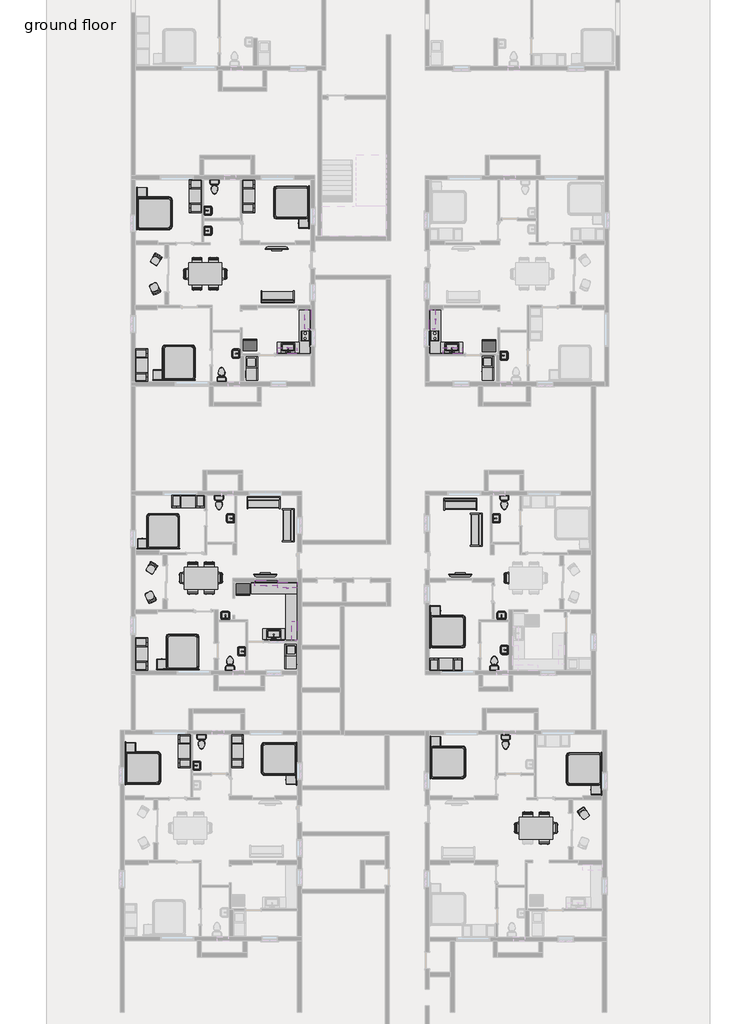
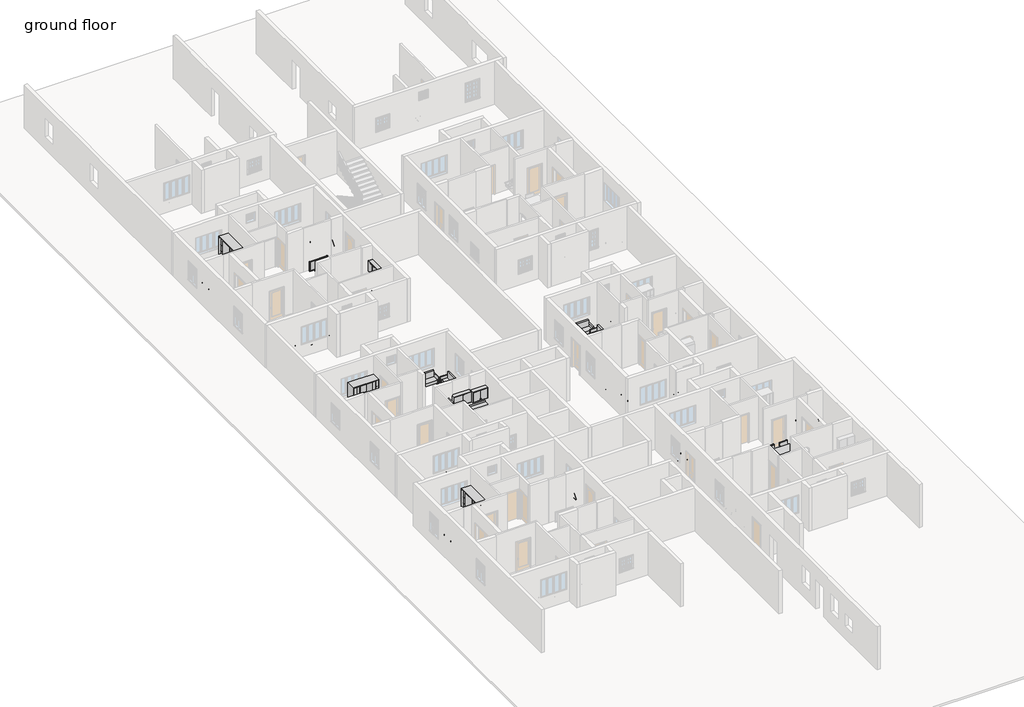
# One storey, part 12 of 16: 77 furniture elements, 22 flow terminals, 11 proxies.
"""IFC4 building model written with IfcOpenShell, lengths in millimetres."""

from ifc_helpers import new_model, si_unit, origin, place, context, project, spatial, transform, mapped, element, save
from components import proxy_84368fe0, proxy_40295e01, proxy_97c73763, proxy_19935bb1, proxy_76352e5b, proxy_1934c8a4, flow_terminal_4d548711, flow_terminal_3ac2e542, flow_terminal_8d9ea526, toilet_domestic_3d_toilet_domestic_3d_ba6479b0, toilet_domestic_3d_toilet_domestic_3d_30431060, bed_design_8999_bed_design_8999_9c973422, bed_design_8999_bed_design_8999_e911dec7, furniture_f87f75a4, furniture_a56de0b1, furniture_5f863b49, furniture_6369f5ad, furniture_97fe820d, furniture_007fecef, chair_task_chair_task_b7f3823b, chair_task_arms_chair_task_arms_fa5a08ef, furniture_deb1c5d1, furniture_78fcf777, furniture_90663022, furniture_1a836c3b, furniture_8d0dc8c9, furniture_49e6720b, furniture_88072bd9, furniture_eb3a3c23, furniture_4fdbbe14, furniture_57f9710a, furniture_0b81fedb, furniture_0bcc43ae, furniture_9929ec1f, furniture_f73e1c42, furniture_4a8f7e85

model = new_model("IFC4")

# Units and contexts
model_context = context("Model", 3, world=origin())
ifc_project = project(units=[si_unit("LENGTHUNIT", "METRE", prefix="MILLI")], contexts=[model_context])

# Site, building, storey
site = spatial("IfcSite", under=ifc_project)
building = spatial("IfcBuilding", under=site)
storey = spatial("IfcBuildingStorey", under=building, Name="ground floor", Elevation=609.6)

# Proxies
placement = place(None, origin())
proxy_shape = proxy_84368fe0(model_context)
element("IfcBuildingElementProxy", 1, Name="Cook Top-2 Unit : 16\" x 22\"", ObjectType="Cook Top-2 Unit : 16\" x 22\"", at=placement, inside=storey, context=model_context, shape_type="MappedRepresentation", body=[
    mapped(proxy_shape, transform((52653.926243, 23760.8750503, 609.6), x_axis=(1.0, 0.0, 0.0), y_axis=(0.0, 1.0, 0.0), z_axis=(0.0, 0.0, 1.0))),
])
proxy_2_shape = proxy_40295e01(model_context)
element("IfcBuildingElementProxy", 2, Name="Cook Top-2 Unit : 16\" x 22\"", ObjectType="Cook Top-2 Unit : 16\" x 22\"", at=placement, inside=storey, context=model_context, shape_type="MappedRepresentation", body=[
    mapped(proxy_2_shape, transform((59966.1312819, 23760.8750503, 609.6), x_axis=(-1.0, 0.0, 0.0), y_axis=(0.0, -1.0, 0.0), z_axis=(0.0, 0.0, 1.0))),
])
proxy_3_shape = proxy_97c73763(model_context)
element("IfcBuildingElementProxy", 3, Name="Dryer : 27\" x 25\" x 35\"", ObjectType="Dryer : 27\" x 25\" x 35\"", at=placement, inside=storey, context=model_context, shape_type="MappedRepresentation", body=[
    mapped(proxy_3_shape, transform((62510.7278279, 22075.5934981, 609.6), x_axis=(0.0, -1.0, 0.0), y_axis=(1.0, 0.0, 0.0), z_axis=(0.0, 0.0, 1.0))),
])
element("IfcBuildingElementProxy", 4, Name="Dryer : 27\" x 25\" x 35\"", ObjectType="Dryer : 27\" x 25\" x 35\"", at=placement, inside=storey, context=model_context, shape_type="MappedRepresentation", body=[
    mapped(proxy_3_shape, transform((49480.5278279, 22050.1934981, 609.6), x_axis=(0.0, -1.0, 0.0), y_axis=(1.0, 0.0, 0.0), z_axis=(0.0, 0.0, 1.0))),
])
element("IfcBuildingElementProxy", 5, Name="Dryer : 27\" x 25\" x 35\"", ObjectType="Dryer : 27\" x 25\" x 35\"", at=placement, inside=storey, context=model_context, shape_type="MappedRepresentation", body=[
    mapped(proxy_3_shape, transform((52244.3504974, 5396.4843277, 609.6), x_axis=(0.0, 1.0, 0.0), y_axis=(-1.0, 0.0, 0.0), z_axis=(0.0, 0.0, 1.0))),
])
proxy_4_shape = proxy_19935bb1(model_context)
element("IfcBuildingElementProxy", 6, Name="Refrigerator-Built-in : 30\" x 24\" LH", ObjectType="Refrigerator-Built-in : 30\" x 24\" LH", at=placement, inside=storey, context=model_context, shape_type="MappedRepresentation", body=[
    mapped(proxy_4_shape, transform((49314.0778826, 9828.1563876, 609.6), x_axis=(1.0, 0.0, 0.0), y_axis=(0.0, 1.0, 0.0), z_axis=(0.0, 0.0, 1.0))),
])
proxy_5_shape = proxy_76352e5b(model_context)
element("IfcBuildingElementProxy", 7, Name="Refrigerator-Built-in : 30\" x 24\" LH", ObjectType="Refrigerator-Built-in : 30\" x 24\" LH", at=placement, inside=storey, context=model_context, shape_type="MappedRepresentation", body=[
    mapped(proxy_5_shape, transform((62882.4552131, 23205.265558, 609.6), x_axis=(1.0, 0.0, 0.0), y_axis=(0.0, 1.0, 0.0), z_axis=(0.0, 0.0, 1.0))),
])
element("IfcBuildingElementProxy", 8, Name="Refrigerator-Built-in : 30\" x 24\" LH", ObjectType="Refrigerator-Built-in : 30\" x 24\" LH", at=placement, inside=storey, context=model_context, shape_type="MappedRepresentation", body=[
    mapped(proxy_5_shape, transform((49699.8552131, 23256.065558, 609.6), x_axis=(1.0, 0.0, 0.0), y_axis=(0.0, 1.0, 0.0), z_axis=(0.0, 0.0, 1.0))),
])
proxy_6_shape = proxy_1934c8a4(model_context)
element("IfcBuildingElementProxy", 9, Name="Washer : 25\" x 25\" x 35\"", ObjectType="Washer : 25\" x 25\" x 35\"", at=placement, inside=storey, context=model_context, shape_type="MappedRepresentation", body=[
    mapped(proxy_6_shape, transform((62546.2392669, 22752.0235103, 609.6), x_axis=(0.0, -1.0, 0.0), y_axis=(1.0, 0.0, 0.0), z_axis=(0.0, 0.0, 1.0))),
])
element("IfcBuildingElementProxy", 10, Name="Washer : 25\" x 25\" x 35\"", ObjectType="Washer : 25\" x 25\" x 35\"", at=placement, inside=storey, context=model_context, shape_type="MappedRepresentation", body=[
    mapped(proxy_6_shape, transform((49516.0392669, 22726.6235103, 609.6), x_axis=(0.0, -1.0, 0.0), y_axis=(1.0, 0.0, 0.0), z_axis=(0.0, 0.0, 1.0))),
])
element("IfcBuildingElementProxy", 11, Name="Washer : 25\" x 25\" x 35\"", ObjectType="Washer : 25\" x 25\" x 35\"", at=placement, inside=storey, context=model_context, shape_type="MappedRepresentation", body=[
    mapped(proxy_6_shape, transform((52203.6619364, 6072.9143399, 609.6), x_axis=(0.0, 1.0, 0.0), y_axis=(-1.0, 0.0, 0.0), z_axis=(0.0, 0.0, 1.0))),
])

# Flow terminals
flow_terminal_shape = flow_terminal_4d548711(model_context)
element("IfcFlowTerminal", 12, ObjectType="Sink Kitchen-Single : 30\" x 21\"", at=placement, inside=storey, context=model_context, shape_type="MappedRepresentation", body=[
    mapped(flow_terminal_shape, transform((51806.0154836, 23119.0104663, 609.6), x_axis=(-1.0, 0.0, 0.0), y_axis=(0.0, -1.0, 0.0), z_axis=(0.0, 0.0, 1.0))),
])
element("IfcFlowTerminal", 13, ObjectType="Sink Kitchen-Single : 30\" x 21\"", at=placement, inside=storey, context=model_context, shape_type="MappedRepresentation", body=[
    mapped(flow_terminal_shape, transform((51016.5809161, 7307.5104663, 609.6), x_axis=(-1.0, 0.0, 0.0), y_axis=(0.0, -1.0, 0.0), z_axis=(0.0, 0.0, 1.0))),
])
flow_terminal_2_shape = flow_terminal_3ac2e542(model_context)
element("IfcFlowTerminal", 14, ObjectType="Sink Kitchen-Single : 30\" x 21\"", at=placement, inside=storey, context=model_context, shape_type="MappedRepresentation", body=[
    mapped(flow_terminal_2_shape, transform((60814.0420413, 23119.0104663, 609.6), x_axis=(1.0, 0.0, 0.0), y_axis=(0.0, 1.0, 0.0), z_axis=(0.0, 0.0, 1.0))),
])
flow_terminal_3_shape = flow_terminal_8d9ea526(model_context)
element("IfcFlowTerminal", 15, ObjectType="Sink Vanity-Square : 20\" x 18\"", at=placement, inside=storey, context=model_context, shape_type="MappedRepresentation", body=[
    mapped(flow_terminal_3_shape, transform((63651.476683, 22681.8758246, 609.6), x_axis=(0.0, 1.0, 0.0), y_axis=(-1.0, 0.0, 0.0), z_axis=(0.0, 0.0, 1.0))),
])
element("IfcFlowTerminal", 16, ObjectType="Sink Vanity-Square : 20\" x 18\"", at=placement, inside=storey, context=model_context, shape_type="MappedRepresentation", body=[
    mapped(flow_terminal_3_shape, transform((63232.376683, 13706.0559785, 609.6), x_axis=(0.0, 1.0, 0.0), y_axis=(-1.0, 0.0, 0.0), z_axis=(0.0, 0.0, 1.0))),
])
element("IfcFlowTerminal", 17, ObjectType="Sink Vanity-Square : 20\" x 18\"", at=placement, inside=storey, context=model_context, shape_type="MappedRepresentation", body=[
    mapped(flow_terminal_3_shape, transform((63582.2705224, 8323.5104663, 609.6), x_axis=(-1.0, 0.0, 0.0), y_axis=(0.0, -1.0, 0.0), z_axis=(0.0, 0.0, 1.0))),
])
element("IfcFlowTerminal", 18, ObjectType="Sink Vanity-Square : 20\" x 18\"", at=placement, inside=storey, context=model_context, shape_type="MappedRepresentation", body=[
    mapped(flow_terminal_3_shape, transform((63773.7858807, 6482.6543057, 609.6), x_axis=(0.0, -1.0, 0.0), y_axis=(1.0, 0.0, 0.0), z_axis=(0.0, 0.0, 1.0))),
])
element("IfcFlowTerminal", 19, ObjectType="Sink Vanity-Square : 20\" x 18\"", at=placement, inside=storey, context=model_context, shape_type="MappedRepresentation", body=[
    mapped(flow_terminal_3_shape, transform((46712.6716441, 66.9997113, 609.6), x_axis=(0.0, 1.0, 0.0), y_axis=(-1.0, 0.0, 0.0), z_axis=(0.0, 0.0, 1.0))),
])
element("IfcFlowTerminal", 20, ObjectType="Sink Vanity-Square : 20\" x 18\"", at=placement, inside=storey, context=model_context, shape_type="MappedRepresentation", body=[
    mapped(flow_terminal_3_shape, transform((49283.8822894, 6399.086689, 609.6), x_axis=(-0.012057146916581555, -0.9999273099621953, 0.0), y_axis=(0.9999273099621953, -0.012057146916581555, 0.0), z_axis=(0.0, 0.0, 1.0))),
])
element("IfcFlowTerminal", 21, ObjectType="Sink Vanity-Square : 20\" x 18\"", at=placement, inside=storey, context=model_context, shape_type="MappedRepresentation", body=[
    mapped(flow_terminal_3_shape, transform((48351.6154836, 8323.5104663, 609.6), x_axis=(-1.0, 0.0, 0.0), y_axis=(0.0, -1.0, 0.0), z_axis=(0.0, 0.0, 1.0))),
])
element("IfcFlowTerminal", 22, ObjectType="Sink Vanity-Square : 20\" x 18\"", at=placement, inside=storey, context=model_context, shape_type="MappedRepresentation", body=[
    mapped(flow_terminal_3_shape, transform((48663.7808419, 13737.4344596, 609.6), x_axis=(0.0, -1.0, 0.0), y_axis=(1.0, 0.0, 0.0), z_axis=(0.0, 0.0, 1.0))),
])
element("IfcFlowTerminal", 23, ObjectType="Sink Vanity-Square : 20\" x 18\"", at=placement, inside=storey, context=model_context, shape_type="MappedRepresentation", body=[
    mapped(flow_terminal_3_shape, transform((48968.5808419, 22827.5543057, 609.6), x_axis=(0.0, -1.0, 0.0), y_axis=(1.0, 0.0, 0.0), z_axis=(0.0, 0.0, 1.0))),
])
element("IfcFlowTerminal", 24, ObjectType="Sink Vanity-Square : 20\" x 18\"", at=placement, inside=storey, context=model_context, shape_type="MappedRepresentation", body=[
    mapped(flow_terminal_3_shape, transform((47322.2716441, 29569.0881062, 609.6), x_axis=(0.0, 1.0, 0.0), y_axis=(-1.0, 0.0, 0.0), z_axis=(0.0, 0.0, 1.0))),
])
element("IfcFlowTerminal", 25, ObjectType="Sink Vanity-Square : 20\" x 18\"", at=placement, inside=storey, context=model_context, shape_type="MappedRepresentation", body=[
    mapped(flow_terminal_3_shape, transform((47322.2716441, 30681.1004564, 609.6), x_axis=(0.0, 1.0, 0.0), y_axis=(-1.0, 0.0, 0.0), z_axis=(0.0, 0.0, 1.0))),
])
toilet_domestic_3d_toilet_domestic_3d_shape = toilet_domestic_3d_toilet_domestic_3d_ba6479b0(model_context)
toilet_domestic_3d_toilet_domestic_3d_2_shape = toilet_domestic_3d_toilet_domestic_3d_30431060(model_context)
element("IfcFlowTerminal", 26, ObjectType="Toilet-Domestic-3D : Toilet-Domestic-3D", at=placement, inside=storey, context=model_context, shape_type="MappedRepresentation", body=[
    mapped(toilet_domestic_3d_toilet_domestic_3d_shape, transform((48129.1248418, 21744.3232288, 609.6), x_axis=(-1.0, 0.0, 0.0), y_axis=(0.0, -1.0, 0.0), z_axis=(0.0, 0.0, 1.0))),
    mapped(toilet_domestic_3d_toilet_domestic_3d_2_shape, transform((48129.1248418, 21744.3232288, 609.6), x_axis=(-1.0, 0.0, 0.0), y_axis=(0.0, -1.0, 0.0), z_axis=(0.0, 0.0, 1.0))),
])
element("IfcFlowTerminal", 27, ObjectType="Toilet-Domestic-3D : Toilet-Domestic-3D", at=placement, inside=storey, context=model_context, shape_type="MappedRepresentation", body=[
    mapped(toilet_domestic_3d_toilet_domestic_3d_shape, transform((47732.676243, 31918.2311741, 609.6), x_axis=(1.0, 0.0, 0.0), y_axis=(0.0, 1.0, 0.0), z_axis=(0.0, 0.0, 1.0))),
    mapped(toilet_domestic_3d_toilet_domestic_3d_2_shape, transform((47732.676243, 31918.2311741, 609.6), x_axis=(1.0, 0.0, 0.0), y_axis=(0.0, 1.0, 0.0), z_axis=(0.0, 0.0, 1.0))),
])
element("IfcFlowTerminal", 28, ObjectType="Toilet-Domestic-3D : Toilet-Domestic-3D", at=placement, inside=storey, context=model_context, shape_type="MappedRepresentation", body=[
    mapped(toilet_domestic_3d_toilet_domestic_3d_shape, transform((47986.676243, 14503.375789, 609.6), x_axis=(1.0, 0.0, 0.0), y_axis=(0.0, 1.0, 0.0), z_axis=(0.0, 0.0, 1.0))),
    mapped(toilet_domestic_3d_toilet_domestic_3d_2_shape, transform((47986.676243, 14503.375789, 609.6), x_axis=(1.0, 0.0, 0.0), y_axis=(0.0, 1.0, 0.0), z_axis=(0.0, 0.0, 1.0))),
])
element("IfcFlowTerminal", 29, ObjectType="Toilet-Domestic-3D : Toilet-Domestic-3D", at=placement, inside=storey, context=model_context, shape_type="MappedRepresentation", body=[
    mapped(toilet_domestic_3d_toilet_domestic_3d_shape, transform((48589.926243, 5815.3678437, 609.6), x_axis=(-1.0, 0.0, 0.0), y_axis=(0.0, -1.0, 0.0), z_axis=(0.0, 0.0, 1.0))),
    mapped(toilet_domestic_3d_toilet_domestic_3d_2_shape, transform((48589.926243, 5815.3678437, 609.6), x_axis=(-1.0, 0.0, 0.0), y_axis=(0.0, -1.0, 0.0), z_axis=(0.0, 0.0, 1.0))),
])
element("IfcFlowTerminal", 30, ObjectType="Toilet-Domestic-3D : Toilet-Domestic-3D", at=placement, inside=storey, context=model_context, shape_type="MappedRepresentation", body=[
    mapped(toilet_domestic_3d_toilet_domestic_3d_shape, transform((63166.5312819, 5818.6610925, 609.6), x_axis=(-1.0, 0.0, 0.0), y_axis=(0.0, -1.0, 0.0), z_axis=(0.0, 0.0, 1.0))),
    mapped(toilet_domestic_3d_toilet_domestic_3d_2_shape, transform((63166.5312819, 5818.6610925, 609.6), x_axis=(-1.0, 0.0, 0.0), y_axis=(0.0, -1.0, 0.0), z_axis=(0.0, 0.0, 1.0))),
])
element("IfcFlowTerminal", 31, ObjectType="Toilet-Domestic-3D : Toilet-Domestic-3D", at=placement, inside=storey, context=model_context, shape_type="MappedRepresentation", body=[
    mapped(toilet_domestic_3d_toilet_domestic_3d_shape, transform((63718.9812819, 14506.6690378, 609.6), x_axis=(1.0, 0.0, 0.0), y_axis=(0.0, 1.0, 0.0), z_axis=(0.0, 0.0, 1.0))),
    mapped(toilet_domestic_3d_toilet_domestic_3d_2_shape, transform((63718.9812819, 14506.6690378, 609.6), x_axis=(1.0, 0.0, 0.0), y_axis=(0.0, 1.0, 0.0), z_axis=(0.0, 0.0, 1.0))),
])
element("IfcFlowTerminal", 32, ObjectType="Toilet-Domestic-3D : Toilet-Domestic-3D", at=placement, inside=storey, context=model_context, shape_type="MappedRepresentation", body=[
    mapped(toilet_domestic_3d_toilet_domestic_3d_shape, transform((63795.1812819, 1292.0926062, 609.6), x_axis=(1.0, 0.0, 0.0), y_axis=(0.0, 1.0, 0.0), z_axis=(0.0, 0.0, 1.0))),
    mapped(toilet_domestic_3d_toilet_domestic_3d_2_shape, transform((63795.1812819, 1292.0926062, 609.6), x_axis=(1.0, 0.0, 0.0), y_axis=(0.0, 1.0, 0.0), z_axis=(0.0, 0.0, 1.0))),
])
element("IfcFlowTerminal", 33, ObjectType="Toilet-Domestic-3D : Toilet-Domestic-3D", at=placement, inside=storey, context=model_context, shape_type="MappedRepresentation", body=[
    mapped(toilet_domestic_3d_toilet_domestic_3d_shape, transform((47021.476243, 1304.7926062, 609.6), x_axis=(1.0, 0.0, 0.0), y_axis=(0.0, 1.0, 0.0), z_axis=(0.0, 0.0, 1.0))),
    mapped(toilet_domestic_3d_toilet_domestic_3d_2_shape, transform((47021.476243, 1304.7926062, 609.6), x_axis=(1.0, 0.0, 0.0), y_axis=(0.0, 1.0, 0.0), z_axis=(0.0, 0.0, 1.0))),
])

# Furniture
bed_design_8999_bed_design_8999_shape = bed_design_8999_bed_design_8999_9c973422(model_context)
bed_design_8999_bed_design_8999_2_shape = bed_design_8999_bed_design_8999_e911dec7(model_context)
element("IfcFurniture", 34, ObjectType="BED_DESIGN_8999 : BED_DESIGN_8999", at=placement, inside=storey, context=model_context, shape_type="MappedRepresentation", body=[
    mapped(bed_design_8999_bed_design_8999_shape, transform((61568.6818649, 7679.8150652, 609.6), x_axis=(0.0, 1.0, 0.0), y_axis=(-1.0, 0.0, 0.0), z_axis=(0.0, 0.0, 1.0))),
    mapped(bed_design_8999_bed_design_8999_2_shape, transform((61568.6818649, 7679.8150652, 609.6), x_axis=(0.0, 1.0, 0.0), y_axis=(-1.0, 0.0, 0.0), z_axis=(0.0, 0.0, 1.0))),
])
element("IfcFurniture", 35, ObjectType="BED_DESIGN_8999 : BED_DESIGN_8999", at=placement, inside=storey, context=model_context, shape_type="MappedRepresentation", body=[
    mapped(bed_design_8999_bed_design_8999_shape, transform((67141.6312819, -302.3613664, 609.6), x_axis=(0.0, -1.0, 0.0), y_axis=(1.0, 0.0, 0.0), z_axis=(0.0, 0.0, 1.0))),
    mapped(bed_design_8999_bed_design_8999_2_shape, transform((67141.6312819, -302.3613664, 609.6), x_axis=(0.0, -1.0, 0.0), y_axis=(1.0, 0.0, 0.0), z_axis=(0.0, 0.0, 1.0))),
])
element("IfcFurniture", 36, ObjectType="BED_DESIGN_8999 : BED_DESIGN_8999", at=placement, inside=storey, context=model_context, shape_type="MappedRepresentation", body=[
    mapped(bed_design_8999_bed_design_8999_shape, transform((61579.0312819, 460.9590685, 609.6), x_axis=(0.0, 1.0, 0.0), y_axis=(-1.0, 0.0, 0.0), z_axis=(0.0, 0.0, 1.0))),
    mapped(bed_design_8999_bed_design_8999_2_shape, transform((61579.0312819, 460.9590685, 609.6), x_axis=(0.0, 1.0, 0.0), y_axis=(-1.0, 0.0, 0.0), z_axis=(0.0, 0.0, 1.0))),
])
element("IfcFurniture", 37, ObjectType="BED_DESIGN_8999 : BED_DESIGN_8999", at=placement, inside=storey, context=model_context, shape_type="MappedRepresentation", body=[
    mapped(bed_design_8999_bed_design_8999_shape, transform((44754.526243, 147.57086, 609.6), x_axis=(0.0, 1.0, 0.0), y_axis=(-1.0, 0.0, 0.0), z_axis=(0.0, 0.0, 1.0))),
    mapped(bed_design_8999_bed_design_8999_2_shape, transform((44754.526243, 147.57086, 609.6), x_axis=(0.0, 1.0, 0.0), y_axis=(-1.0, 0.0, 0.0), z_axis=(0.0, 0.0, 1.0))),
])
element("IfcFurniture", 38, ObjectType="BED_DESIGN_8999 : BED_DESIGN_8999", at=placement, inside=storey, context=model_context, shape_type="MappedRepresentation", body=[
    mapped(bed_design_8999_bed_design_8999_shape, transform((50317.126243, 256.4386336, 609.6), x_axis=(0.0, -1.0, 0.0), y_axis=(1.0, 0.0, 0.0), z_axis=(0.0, 0.0, 1.0))),
    mapped(bed_design_8999_bed_design_8999_2_shape, transform((50317.126243, 256.4386336, 609.6), x_axis=(0.0, -1.0, 0.0), y_axis=(1.0, 0.0, 0.0), z_axis=(0.0, 0.0, 1.0))),
])
element("IfcFurniture", 39, ObjectType="BED_DESIGN_8999 : BED_DESIGN_8999", at=placement, inside=storey, context=model_context, shape_type="MappedRepresentation", body=[
    mapped(bed_design_8999_bed_design_8999_shape, transform((45770.526243, 7332.9156483, 609.6), x_axis=(-1.0, 0.0, 0.0), y_axis=(0.0, -1.0, 0.0), z_axis=(0.0, 0.0, 1.0))),
    mapped(bed_design_8999_bed_design_8999_2_shape, transform((45770.526243, 7332.9156483, 609.6), x_axis=(-1.0, 0.0, 0.0), y_axis=(0.0, -1.0, 0.0), z_axis=(0.0, 0.0, 1.0))),
])
element("IfcFurniture", 40, ObjectType="BED_DESIGN_8999 : BED_DESIGN_8999", at=placement, inside=storey, context=model_context, shape_type="MappedRepresentation", body=[
    mapped(bed_design_8999_bed_design_8999_shape, transform((44703.726243, 13985.3658272, 609.6), x_axis=(-1.0, 0.0, 0.0), y_axis=(0.0, -1.0, 0.0), z_axis=(0.0, 0.0, 1.0))),
    mapped(bed_design_8999_bed_design_8999_2_shape, transform((44703.726243, 13985.3658272, 609.6), x_axis=(-1.0, 0.0, 0.0), y_axis=(0.0, -1.0, 0.0), z_axis=(0.0, 0.0, 1.0))),
])
element("IfcFurniture", 41, ObjectType="BED_DESIGN_8999 : BED_DESIGN_8999", at=placement, inside=storey, context=model_context, shape_type="MappedRepresentation", body=[
    mapped(bed_design_8999_bed_design_8999_shape, transform((45567.326243, 23281.7658272, 609.6), x_axis=(-1.0, 0.0, 0.0), y_axis=(0.0, -1.0, 0.0), z_axis=(0.0, 0.0, 1.0))),
    mapped(bed_design_8999_bed_design_8999_2_shape, transform((45567.326243, 23281.7658272, 609.6), x_axis=(-1.0, 0.0, 0.0), y_axis=(0.0, -1.0, 0.0), z_axis=(0.0, 0.0, 1.0))),
])
element("IfcFurniture", 42, ObjectType="BED_DESIGN_8999 : BED_DESIGN_8999", at=placement, inside=storey, context=model_context, shape_type="MappedRepresentation", body=[
    mapped(bed_design_8999_bed_design_8999_shape, transform((51002.925481, 30946.2150652, 609.6), x_axis=(0.0, -1.0, 0.0), y_axis=(1.0, 0.0, 0.0), z_axis=(0.0, 0.0, 1.0))),
    mapped(bed_design_8999_bed_design_8999_2_shape, transform((51002.925481, 30946.2150652, 609.6), x_axis=(0.0, -1.0, 0.0), y_axis=(1.0, 0.0, 0.0), z_axis=(0.0, 0.0, 1.0))),
])
element("IfcFurniture", 43, ObjectType="BED_DESIGN_8999 : BED_DESIGN_8999", at=placement, inside=storey, context=model_context, shape_type="MappedRepresentation", body=[
    mapped(bed_design_8999_bed_design_8999_shape, transform((45389.526243, 30749.2272014, 609.6), x_axis=(0.0, 1.0, 0.0), y_axis=(-1.0, 0.0, 0.0), z_axis=(0.0, 0.0, 1.0))),
    mapped(bed_design_8999_bed_design_8999_2_shape, transform((45389.526243, 30749.2272014, 609.6), x_axis=(0.0, 1.0, 0.0), y_axis=(-1.0, 0.0, 0.0), z_axis=(0.0, 0.0, 1.0))),
])
furniture_shape = furniture_f87f75a4(model_context)
element("IfcFurniture", 44, ObjectType="Base Cabinet-Combo01 : 30\"", at=placement, inside=storey, context=model_context, shape_type="MappedRepresentation", body=[
    mapped(furniture_shape, transform((53034.926243, 24888.4160974, 609.6), x_axis=(0.0, -1.0, 0.0), y_axis=(1.0, 0.0, 0.0), z_axis=(0.0, 0.0, 1.0))),
])
element("IfcFurniture", 45, ObjectType="Base Cabinet-Combo01 : 30\"", at=placement, inside=storey, context=model_context, shape_type="MappedRepresentation", body=[
    mapped(furniture_shape, transform((53034.926243, 24126.4160974, 609.6), x_axis=(0.0, -1.0, 0.0), y_axis=(1.0, 0.0, 0.0), z_axis=(0.0, 0.0, 1.0))),
])
element("IfcFurniture", 46, ObjectType="Base Cabinet-Combo01 : 30\"", at=placement, inside=storey, context=model_context, shape_type="MappedRepresentation", body=[
    mapped(furniture_shape, transform((52311.026243, 8314.9160974, 609.6), x_axis=(0.0, -1.0, 0.0), y_axis=(1.0, 0.0, 0.0), z_axis=(0.0, 0.0, 1.0))),
])
furniture_2_shape = furniture_a56de0b1(model_context)
element("IfcFurniture", 47, ObjectType="Base Cabinet-Combo01 : 30\"", at=placement, inside=storey, context=model_context, shape_type="MappedRepresentation", body=[
    mapped(furniture_2_shape, transform((59585.1312819, 24888.4160974, 609.6), x_axis=(0.0, -1.0, 0.0), y_axis=(1.0, 0.0, 0.0), z_axis=(0.0, 0.0, 1.0))),
])
element("IfcFurniture", 48, ObjectType="Base Cabinet-Combo01 : 30\"", at=placement, inside=storey, context=model_context, shape_type="MappedRepresentation", body=[
    mapped(furniture_2_shape, transform((59585.1312819, 24126.4160974, 609.6), x_axis=(0.0, -1.0, 0.0), y_axis=(1.0, 0.0, 0.0), z_axis=(0.0, 0.0, 1.0))),
])
furniture_3_shape = furniture_5f863b49(model_context)
element("IfcFurniture", 49, ObjectType="Base Cabinet-Combo01 : 30\" 3", at=placement, inside=storey, context=model_context, shape_type="MappedRepresentation", body=[
    mapped(furniture_3_shape, transform((50576.8488369, 10315.0650652, 609.6), x_axis=(1.0, 0.0, 0.0), y_axis=(0.0, 1.0, 0.0), z_axis=(0.0, 0.0, 1.0))),
])
furniture_4_shape = furniture_6369f5ad(model_context)
element("IfcFurniture", 50, ObjectType="Base Cabinet-Combo01 : 30\" 4", at=placement, inside=storey, context=model_context, shape_type="MappedRepresentation", body=[
    mapped(furniture_4_shape, transform((52311.026243, 9000.7160974, 609.6), x_axis=(0.0, -1.0, 0.0), y_axis=(1.0, 0.0, 0.0), z_axis=(0.0, 0.0, 1.0))),
])
furniture_5_shape = furniture_97fe820d(model_context)
element("IfcFurniture", 51, ObjectType="Base Cabinet-Corner Unit-Square : 36\"", at=placement, inside=storey, context=model_context, shape_type="MappedRepresentation", body=[
    mapped(furniture_5_shape, transform((53034.926243, 23338.3915073, 609.6), x_axis=(0.0, -1.0, 0.0), y_axis=(1.0, 0.0, 0.0), z_axis=(0.0, 0.0, 1.0))),
])
element("IfcFurniture", 52, ObjectType="Base Cabinet-Corner Unit-Square : 36\"", at=placement, inside=storey, context=model_context, shape_type="MappedRepresentation", body=[
    mapped(furniture_5_shape, transform((52311.026243, 7526.8915073, 609.6), x_axis=(0.0, -1.0, 0.0), y_axis=(1.0, 0.0, 0.0), z_axis=(0.0, 0.0, 1.0))),
])
element("IfcFurniture", 53, ObjectType="Base Cabinet-Corner Unit-Square : 36\"", at=placement, inside=storey, context=model_context, shape_type="MappedRepresentation", body=[
    mapped(furniture_5_shape, transform((51784.2885381, 10204.3533925, 609.6), x_axis=(1.0, 0.0, 0.0), y_axis=(0.0, 1.0, 0.0), z_axis=(0.0, 0.0, 1.0))),
])
furniture_6_shape = furniture_007fecef(model_context)
element("IfcFurniture", 54, ObjectType="Base Cabinet-Corner Unit-Square : 36\"", at=placement, inside=storey, context=model_context, shape_type="MappedRepresentation", body=[
    mapped(furniture_6_shape, transform((59585.1312819, 23338.3915073, 609.6), x_axis=(0.0, -1.0, 0.0), y_axis=(1.0, 0.0, 0.0), z_axis=(0.0, 0.0, 1.0))),
])
chair_task_chair_task_shape = chair_task_chair_task_b7f3823b(model_context)
element("IfcFurniture", 55, ObjectType="Chair-Task : Chair-Task", at=placement, inside=storey, context=model_context, shape_type="MappedRepresentation", body=[
    mapped(chair_task_chair_task_shape, transform((46631.8073922, 26580.5700511, 609.6), x_axis=(1.0, 0.0, 0.0), y_axis=(0.0, 1.0, 0.0), z_axis=(0.0, 0.0, 1.0))),
])
element("IfcFurniture", 56, ObjectType="Chair-Task : Chair-Task", at=placement, inside=storey, context=model_context, shape_type="MappedRepresentation", body=[
    mapped(chair_task_chair_task_shape, transform((46913.7890315, 27837.6618544, 609.6), x_axis=(-1.0, 0.0, 0.0), y_axis=(0.0, -1.0, 0.0), z_axis=(0.0, 0.0, 1.0))),
])
element("IfcFurniture", 57, ObjectType="Chair-Task : Chair-Task", at=placement, inside=storey, context=model_context, shape_type="MappedRepresentation", body=[
    mapped(chair_task_chair_task_shape, transform((47546.2073922, 26580.5700511, 609.6), x_axis=(1.0, 0.0, 0.0), y_axis=(0.0, 1.0, 0.0), z_axis=(0.0, 0.0, 1.0))),
])
element("IfcFurniture", 58, ObjectType="Chair-Task : Chair-Task", at=placement, inside=storey, context=model_context, shape_type="MappedRepresentation", body=[
    mapped(chair_task_chair_task_shape, transform((47828.1890315, 27837.6618544, 609.6), x_axis=(-1.0, 0.0, 0.0), y_axis=(0.0, -1.0, 0.0), z_axis=(0.0, 0.0, 1.0))),
])
element("IfcFurniture", 59, ObjectType="Chair-Task : Chair-Task", at=placement, inside=storey, context=model_context, shape_type="MappedRepresentation", body=[
    mapped(chair_task_chair_task_shape, transform((46391.5354234, 9800.8191635, 609.6), x_axis=(1.0, 0.0, 0.0), y_axis=(0.0, 1.0, 0.0), z_axis=(0.0, 0.0, 1.0))),
])
element("IfcFurniture", 60, ObjectType="Chair-Task : Chair-Task", at=placement, inside=storey, context=model_context, shape_type="MappedRepresentation", body=[
    mapped(chair_task_chair_task_shape, transform((46673.5170627, 11057.9109668, 609.6), x_axis=(-1.0, 0.0, 0.0), y_axis=(0.0, -1.0, 0.0), z_axis=(0.0, 0.0, 1.0))),
])
element("IfcFurniture", 61, ObjectType="Chair-Task : Chair-Task", at=placement, inside=storey, context=model_context, shape_type="MappedRepresentation", body=[
    mapped(chair_task_chair_task_shape, transform((47305.9354234, 9800.8191635, 609.6), x_axis=(1.0, 0.0, 0.0), y_axis=(0.0, 1.0, 0.0), z_axis=(0.0, 0.0, 1.0))),
])
element("IfcFurniture", 62, ObjectType="Chair-Task : Chair-Task", at=placement, inside=storey, context=model_context, shape_type="MappedRepresentation", body=[
    mapped(chair_task_chair_task_shape, transform((47587.9170627, 11057.9109668, 609.6), x_axis=(-1.0, 0.0, 0.0), y_axis=(0.0, -1.0, 0.0), z_axis=(0.0, 0.0, 1.0))),
])
element("IfcFurniture", 63, ObjectType="Chair-Task : Chair-Task", at=placement, inside=storey, context=model_context, shape_type="MappedRepresentation", body=[
    mapped(chair_task_chair_task_shape, transform((65155.3721015, -2732.4930795, 609.6), x_axis=(-1.0, 0.0, 0.0), y_axis=(0.0, -1.0, 0.0), z_axis=(0.0, 0.0, 1.0))),
])
element("IfcFurniture", 64, ObjectType="Chair-Task : Chair-Task", at=placement, inside=storey, context=model_context, shape_type="MappedRepresentation", body=[
    mapped(chair_task_chair_task_shape, transform((65787.7904622, -3989.5848828, 609.6), x_axis=(1.0, 0.0, 0.0), y_axis=(0.0, 1.0, 0.0), z_axis=(0.0, 0.0, 1.0))),
])
element("IfcFurniture", 65, ObjectType="Chair-Task : Chair-Task", at=placement, inside=storey, context=model_context, shape_type="MappedRepresentation", body=[
    mapped(chair_task_chair_task_shape, transform((66069.7721015, -2732.4930795, 609.6), x_axis=(-1.0, 0.0, 0.0), y_axis=(0.0, -1.0, 0.0), z_axis=(0.0, 0.0, 1.0))),
])
chair_task_arms_chair_task_arms_shape = chair_task_arms_chair_task_arms_fa5a08ef(model_context)
element("IfcFurniture", 66, ObjectType="Chair-Task Arms : Chair-Task Arms", at=placement, inside=storey, context=model_context, shape_type="MappedRepresentation", body=[
    mapped(chair_task_arms_chair_task_arms_shape, transform((48163.3441135, 27068.1251331, 609.6), x_axis=(0.0, 1.0, 0.0), y_axis=(-1.0, 0.0, 0.0), z_axis=(0.0, 0.0, 1.0))),
])
element("IfcFurniture", 67, ObjectType="Chair-Task Arms : Chair-Task Arms", at=placement, inside=storey, context=model_context, shape_type="MappedRepresentation", body=[
    mapped(chair_task_arms_chair_task_arms_shape, transform((46296.6523102, 27350.1067724, 609.6), x_axis=(0.0, -1.0, 0.0), y_axis=(1.0, 0.0, 0.0), z_axis=(0.0, 0.0, 1.0))),
])
element("IfcFurniture", 68, ObjectType="Chair-Task Arms : Chair-Task Arms", at=placement, inside=storey, context=model_context, shape_type="MappedRepresentation", body=[
    mapped(chair_task_arms_chair_task_arms_shape, transform((47923.0721447, 10288.3742455, 609.6), x_axis=(0.0, 1.0, 0.0), y_axis=(-1.0, 0.0, 0.0), z_axis=(0.0, 0.0, 1.0))),
])
element("IfcFurniture", 69, ObjectType="Chair-Task Arms : Chair-Task Arms", at=placement, inside=storey, context=model_context, shape_type="MappedRepresentation", body=[
    mapped(chair_task_arms_chair_task_arms_shape, transform((46056.3803414, 10570.3558848, 609.6), x_axis=(0.0, -1.0, 0.0), y_axis=(1.0, 0.0, 0.0), z_axis=(0.0, 0.0, 1.0))),
])
element("IfcFurniture", 70, ObjectType="Chair-Task Arms : Chair-Task Arms", at=placement, inside=storey, context=model_context, shape_type="MappedRepresentation", body=[
    mapped(chair_task_arms_chair_task_arms_shape, transform((63973.0853802, 10570.3558848, 609.6), x_axis=(0.0, -1.0, 0.0), y_axis=(1.0, 0.0, 0.0), z_axis=(0.0, 0.0, 1.0))),
])
element("IfcFurniture", 71, ObjectType="Chair-Task Arms : Chair-Task Arms", at=placement, inside=storey, context=model_context, shape_type="MappedRepresentation", body=[
    mapped(chair_task_arms_chair_task_arms_shape, transform((66404.9271835, -3502.0298008, 609.6), x_axis=(0.0, 1.0, 0.0), y_axis=(-1.0, 0.0, 0.0), z_axis=(0.0, 0.0, 1.0))),
])
element("IfcFurniture", 72, ObjectType="Chair-Task Arms : Chair-Task Arms", at=placement, inside=storey, context=model_context, shape_type="MappedRepresentation", body=[
    mapped(chair_task_arms_chair_task_arms_shape, transform((64538.2353802, -3220.0481615, 609.6), x_axis=(0.0, -1.0, 0.0), y_axis=(1.0, 0.0, 0.0), z_axis=(0.0, 0.0, 1.0))),
])
furniture_7_shape = furniture_deb1c5d1(model_context)
element("IfcFurniture", 73, ObjectType="Counter Top : 24\" Depth", at=placement, inside=storey, context=model_context, shape_type="MappedRepresentation", body=[
    mapped(furniture_7_shape, transform((53034.926243, 24049.5915073, 609.6), x_axis=(0.0, -1.0, 0.0), y_axis=(1.0, 0.0, 0.0), z_axis=(0.0, 0.0, 1.0))),
])
furniture_8_shape = furniture_78fcf777(model_context)
element("IfcFurniture", 74, ObjectType="Counter Top : 24\" Depth", at=placement, inside=storey, context=model_context, shape_type="MappedRepresentation", body=[
    mapped(furniture_8_shape, transform((59585.1312819, 24049.5915073, 609.6), x_axis=(0.0, -1.0, 0.0), y_axis=(1.0, 0.0, 0.0), z_axis=(0.0, 0.0, 1.0))),
])
furniture_9_shape = furniture_90663022(model_context)
element("IfcFurniture", 75, ObjectType="Counter Top : 24\" Depth", at=placement, inside=storey, context=model_context, shape_type="MappedRepresentation", body=[
    mapped(furniture_9_shape, transform((52311.026243, 8365.3027701, 609.6), x_axis=(0.0, -1.0, 0.0), y_axis=(1.0, 0.0, 0.0), z_axis=(0.0, 0.0, 1.0))),
])
furniture_10_shape = furniture_1a836c3b(model_context)
element("IfcFurniture", 76, ObjectType="Counter Top : 24\" Depth", at=placement, inside=storey, context=model_context, shape_type="MappedRepresentation", body=[
    mapped(furniture_10_shape, transform((50954.5160423, 10200.7650652, 609.6), x_axis=(1.0, 0.0, 0.0), y_axis=(0.0, 1.0, 0.0), z_axis=(0.0, 0.0, 1.0))),
])
furniture_11_shape = furniture_8d0dc8c9(model_context)
element("IfcFurniture", 77, ObjectType="Counter Top w Sink Hole : 24\" Depth", at=placement, inside=storey, context=model_context, shape_type="MappedRepresentation", body=[
    mapped(furniture_11_shape, transform((51199.4639479, 22811.8650652, 609.6), x_axis=(-1.0, 0.0, 0.0), y_axis=(0.0, -1.0, 0.0), z_axis=(0.0, 0.0, 1.0))),
])
element("IfcFurniture", 78, ObjectType="Counter Top w Sink Hole : 24\" Depth", at=placement, inside=storey, context=model_context, shape_type="MappedRepresentation", body=[
    mapped(furniture_11_shape, transform((50410.0293805, 7000.3650652, 609.6), x_axis=(-1.0, 0.0, 0.0), y_axis=(0.0, -1.0, 0.0), z_axis=(0.0, 0.0, 1.0))),
])
furniture_12_shape = furniture_49e6720b(model_context)
element("IfcFurniture", 79, ObjectType="Counter Top w Sink Hole : 24\" Depth", at=placement, inside=storey, context=model_context, shape_type="MappedRepresentation", body=[
    mapped(furniture_12_shape, transform((61420.5935769, 22811.8650652, 609.6), x_axis=(1.0, 0.0, 0.0), y_axis=(0.0, 1.0, 0.0), z_axis=(0.0, 0.0, 1.0))),
])
furniture_13_shape = furniture_88072bd9(model_context)
element("IfcFurniture", 80, ObjectType="Entertainment Center : 72\" x 72\" x 24\"", at=placement, inside=storey, context=model_context, shape_type="MappedRepresentation", body=[
    mapped(furniture_13_shape, transform((60499.5312819, 5222.3650652, 609.6), x_axis=(-1.0, 0.0, 0.0), y_axis=(0.0, -1.0, 0.0), z_axis=(0.0, 0.0, 1.0))),
])
element("IfcFurniture", 81, ObjectType="Entertainment Center : 72\" x 72\" x 24\"", at=placement, inside=storey, context=model_context, shape_type="MappedRepresentation", body=[
    mapped(furniture_13_shape, transform((46519.826243, 872.3886336, 609.6), x_axis=(0.0, -1.0, 0.0), y_axis=(1.0, 0.0, 0.0), z_axis=(0.0, 0.0, 1.0))),
])
element("IfcFurniture", 82, ObjectType="Entertainment Center : 72\" x 72\" x 24\"", at=placement, inside=storey, context=model_context, shape_type="MappedRepresentation", body=[
    mapped(furniture_13_shape, transform((48551.826243, 872.3886336, 609.6), x_axis=(0.0, 1.0, 0.0), y_axis=(-1.0, 0.0, 0.0), z_axis=(0.0, 0.0, 1.0))),
])
element("IfcFurniture", 83, ObjectType="Entertainment Center : 72\" x 72\" x 24\"", at=placement, inside=storey, context=model_context, shape_type="MappedRepresentation", body=[
    mapped(furniture_13_shape, transform((43268.626243, 6235.0718163, 609.6), x_axis=(0.0, 1.0, 0.0), y_axis=(-1.0, 0.0, 0.0), z_axis=(0.0, 0.0, 1.0))),
])
element("IfcFurniture", 84, ObjectType="Entertainment Center : 72\" x 72\" x 24\"", at=placement, inside=storey, context=model_context, shape_type="MappedRepresentation", body=[
    mapped(furniture_13_shape, transform((46291.226243, 15099.6718163, 609.6), x_axis=(1.0, 0.0, 0.0), y_axis=(0.0, 1.0, 0.0), z_axis=(0.0, 0.0, 1.0))),
])
element("IfcFurniture", 85, ObjectType="Entertainment Center : 72\" x 72\" x 24\"", at=placement, inside=storey, context=model_context, shape_type="MappedRepresentation", body=[
    mapped(furniture_13_shape, transform((43268.626243, 22164.0272014, 609.6), x_axis=(0.0, 1.0, 0.0), y_axis=(-1.0, 0.0, 0.0), z_axis=(0.0, 0.0, 1.0))),
])
element("IfcFurniture", 86, ObjectType="Entertainment Center : 72\" x 72\" x 24\"", at=placement, inside=storey, context=model_context, shape_type="MappedRepresentation", body=[
    mapped(furniture_13_shape, transform((47129.426243, 31498.5272014, 609.6), x_axis=(0.0, -1.0, 0.0), y_axis=(1.0, 0.0, 0.0), z_axis=(0.0, 0.0, 1.0))),
])
element("IfcFurniture", 87, ObjectType="Entertainment Center : 72\" x 72\" x 24\"", at=placement, inside=storey, context=model_context, shape_type="MappedRepresentation", body=[
    mapped(furniture_13_shape, transform((49161.426243, 31498.5272014, 609.6), x_axis=(0.0, 1.0, 0.0), y_axis=(-1.0, 0.0, 0.0), z_axis=(0.0, 0.0, 1.0))),
])
furniture_14_shape = furniture_eb3a3c23(model_context)
element("IfcFurniture", 88, ObjectType="Seating-Auditorium : 18\" x 24\" x 30\"", at=placement, inside=storey, context=model_context, shape_type="MappedRepresentation", body=[
    mapped(furniture_14_shape, transform((44751.7812625, 28092.7068331, 609.6), x_axis=(-0.8660254037844514, 0.499999999999978, 0.0), y_axis=(-0.499999999999978, -0.8660254037844514, 0.0), z_axis=(0.0, 0.0, 1.0))),
])
element("IfcFurniture", 89, ObjectType="Seating-Auditorium : 18\" x 24\" x 30\"", at=placement, inside=storey, context=model_context, shape_type="MappedRepresentation", body=[
    mapped(furniture_14_shape, transform((44391.6003424, 26141.477646, 609.6), x_axis=(0.8974056171641766, 0.4412064803265965, 0.0), y_axis=(-0.4412064803265965, 0.8974056171641766, 0.0), z_axis=(0.0, 0.0, 1.0))),
])
element("IfcFurniture", 90, ObjectType="Seating-Auditorium : 18\" x 24\" x 30\"", at=placement, inside=storey, context=model_context, shape_type="MappedRepresentation", body=[
    mapped(furniture_14_shape, transform((44508.5552699, 11076.4450487, 609.6), x_axis=(-0.8660254037844514, 0.499999999999978, 0.0), y_axis=(-0.499999999999978, -0.8660254037844514, 0.0), z_axis=(0.0, 0.0, 1.0))),
])
element("IfcFurniture", 91, ObjectType="Seating-Auditorium : 18\" x 24\" x 30\"", at=placement, inside=storey, context=model_context, shape_type="MappedRepresentation", body=[
    mapped(furniture_14_shape, transform((44148.3743498, 9125.2158615, 609.6), x_axis=(0.8974056171641766, 0.4412064803265965, 0.0), y_axis=(-0.4412064803265965, 0.8974056171641766, 0.0), z_axis=(0.0, 0.0, 1.0))),
])
furniture_15_shape = furniture_4fdbbe14(model_context)
element("IfcFurniture", 92, ObjectType="Seating-Auditorium : 18\" x 24\" x 30\"", at=placement, inside=storey, context=model_context, shape_type="MappedRepresentation", body=[
    mapped(furniture_15_shape, transform((67839.7044741, -2479.9709422, 609.6), x_axis=(0.8090169943749673, 0.5877852522924457, 0.0), y_axis=(-0.5877852522924457, 0.8090169943749673, 0.0), z_axis=(0.0, 0.0, 1.0))),
])
furniture_16_shape = furniture_57f9710a(model_context)
element("IfcFurniture", 93, ObjectType="Sofa : 72\"", at=placement, inside=storey, context=model_context, shape_type="MappedRepresentation", body=[
    mapped(furniture_16_shape, transform((61227.8770053, 14359.9109668, 609.6), x_axis=(1.0, 0.0, 0.0), y_axis=(0.0, 1.0, 0.0), z_axis=(0.0, 0.0, 1.0))),
])
element("IfcFurniture", 94, ObjectType="Sofa : 72\"", at=placement, inside=storey, context=model_context, shape_type="MappedRepresentation", body=[
    mapped(furniture_16_shape, transform((62019.9156717, 13160.385557, 609.6), x_axis=(0.0, -1.0, 0.0), y_axis=(1.0, 0.0, 0.0), z_axis=(0.0, 0.0, 1.0))),
])
element("IfcFurniture", 95, ObjectType="Sofa : 72\"", at=placement, inside=storey, context=model_context, shape_type="MappedRepresentation", body=[
    mapped(furniture_16_shape, transform((51654.1884934, 13409.1079164, 609.6), x_axis=(0.0, -1.0, 0.0), y_axis=(1.0, 0.0, 0.0), z_axis=(0.0, 0.0, 1.0))),
])
element("IfcFurniture", 96, ObjectType="Sofa : 72\"", at=placement, inside=storey, context=model_context, shape_type="MappedRepresentation", body=[
    mapped(furniture_16_shape, transform((50373.7557512, 14432.817718, 609.6), x_axis=(1.0, 0.0, 0.0), y_axis=(0.0, 1.0, 0.0), z_axis=(0.0, 0.0, 1.0))),
])
element("IfcFurniture", 97, ObjectType="Sofa : 72\"", at=placement, inside=storey, context=model_context, shape_type="MappedRepresentation", body=[
    mapped(furniture_16_shape, transform((51285.9748937, 26091.0193745, 609.6), x_axis=(-0.9999999999999946, -1.0543434768966989e-07, 0.0), y_axis=(1.0543434768966989e-07, -0.9999999999999946, 0.0), z_axis=(0.0, 0.0, 1.0))),
])
furniture_17_shape = furniture_0b81fedb(model_context)
element("IfcFurniture", 98, ObjectType="TV - Flat Screen : 50\"", at=placement, inside=storey, context=model_context, shape_type="MappedRepresentation", body=[
    mapped(furniture_17_shape, transform((51171.9707572, 28640.3330139, 609.6), x_axis=(1.0, 0.0, 0.0), y_axis=(0.0, 1.0, 0.0), z_axis=(0.0, 0.0, 1.0))),
])
element("IfcFurniture", 99, ObjectType="TV - Flat Screen : 50\"", at=placement, inside=storey, context=model_context, shape_type="MappedRepresentation", body=[
    mapped(furniture_17_shape, transform((61294.302983, 10566.9202336, 609.6), x_axis=(-1.0, 0.0, 0.0), y_axis=(0.0, -1.0, 0.0), z_axis=(0.0, 0.0, 1.0))),
])
element("IfcFurniture", 100, ObjectType="TV - Flat Screen : 50\"", at=placement, inside=storey, context=model_context, shape_type="MappedRepresentation", body=[
    mapped(furniture_17_shape, transform((50541.7817289, 10566.9202336, 609.6), x_axis=(-1.0, 0.0, 0.0), y_axis=(0.0, -1.0, 0.0), z_axis=(0.0, 0.0, 1.0))),
])
furniture_18_shape = furniture_0bcc43ae(model_context)
element("IfcFurniture", 101, ObjectType="Table-Conference2 w Chairs : 48\" x 144\"", at=placement, inside=storey, context=model_context, shape_type="MappedRepresentation", body=[
    mapped(furniture_18_shape, transform((47229.9982118, 27209.1159527, 609.6), x_axis=(-1.0, 0.0, 0.0), y_axis=(0.0, -1.0, 0.0), z_axis=(0.0, 0.0, 1.0))),
])
element("IfcFurniture", 102, ObjectType="Table-Conference2 w Chairs : 48\" x 144\"", at=placement, inside=storey, context=model_context, shape_type="MappedRepresentation", body=[
    mapped(furniture_18_shape, transform((46989.726243, 10429.3650652, 609.6), x_axis=(-1.0, 0.0, 0.0), y_axis=(0.0, -1.0, 0.0), z_axis=(0.0, 0.0, 1.0))),
])
element("IfcFurniture", 103, ObjectType="Table-Conference2 w Chairs : 48\" x 144\"", at=placement, inside=storey, context=model_context, shape_type="MappedRepresentation", body=[
    mapped(furniture_18_shape, transform((65471.5812819, -3361.0389812, 609.6), x_axis=(-1.0, 0.0, 0.0), y_axis=(0.0, -1.0, 0.0), z_axis=(0.0, 0.0, 1.0))),
])
furniture_19_shape = furniture_9929ec1f(model_context)
element("IfcFurniture", 104, ObjectType="Upper Cabinet-Double Door-Wall : 42\"", at=placement, inside=storey, context=model_context, shape_type="MappedRepresentation", body=[
    mapped(furniture_19_shape, transform((59470.8312819, 24721.236228, 609.6), x_axis=(0.0, -1.0, 0.0), y_axis=(1.0, 0.0, 0.0), z_axis=(0.0, 0.0, 1.0))),
])
element("IfcFurniture", 105, ObjectType="Upper Cabinet-Double Door-Wall : 42\"", at=placement, inside=storey, context=model_context, shape_type="MappedRepresentation", body=[
    mapped(furniture_19_shape, transform((53149.226243, 24661.6939024, 609.6), x_axis=(0.0, 1.0, 0.0), y_axis=(-1.0, 0.0, 0.0), z_axis=(0.0, 0.0, 1.0))),
])
element("IfcFurniture", 106, ObjectType="Upper Cabinet-Double Door-Wall : 42\"", at=placement, inside=storey, context=model_context, shape_type="MappedRepresentation", body=[
    mapped(furniture_19_shape, transform((51793.7577046, 10315.0650652, 609.6), x_axis=(-1.0, 0.0, 0.0), y_axis=(0.0, -1.0, 0.0), z_axis=(0.0, 0.0, 1.0))),
])
element("IfcFurniture", 107, ObjectType="Upper Cabinet-Double Door-Wall : 42\"", at=placement, inside=storey, context=model_context, shape_type="MappedRepresentation", body=[
    mapped(furniture_19_shape, transform((52425.326243, 7497.6439024, 609.6), x_axis=(0.0, 1.0, 0.0), y_axis=(-1.0, 0.0, 0.0), z_axis=(0.0, 0.0, 1.0))),
])
furniture_20_shape = furniture_f73e1c42(model_context)
element("IfcFurniture", 108, ObjectType="Upper Cabinet-Double Door-Wall : 42\"", at=placement, inside=storey, context=model_context, shape_type="MappedRepresentation", body=[
    mapped(furniture_20_shape, transform((60850.7601191, 22754.7150652, 609.6), x_axis=(1.0, 0.0, 0.0), y_axis=(0.0, 1.0, 0.0), z_axis=(0.0, 0.0, 1.0))),
])
element("IfcFurniture", 109, ObjectType="Upper Cabinet-Double Door-Wall : 42\"", at=placement, inside=storey, context=model_context, shape_type="MappedRepresentation", body=[
    mapped(furniture_20_shape, transform((51722.4550802, 22754.7150652, 609.6), x_axis=(1.0, 0.0, 0.0), y_axis=(0.0, 1.0, 0.0), z_axis=(0.0, 0.0, 1.0))),
])
furniture_21_shape = furniture_4a8f7e85(model_context)
element("IfcFurniture", 110, ObjectType="Upper Cabinet-Double Door-Wall : 42\" 2", at=placement, inside=storey, context=model_context, shape_type="MappedRepresentation", body=[
    mapped(furniture_21_shape, transform((50619.2848585, 10372.2150652, 609.6), x_axis=(-1.0, 0.0, 0.0), y_axis=(0.0, -1.0, 0.0), z_axis=(0.0, 0.0, 1.0))),
])

save(model, "model.ifc")

# Revit data of these elements
# Type "Cook Top-2 Unit : 16\" x 22\""
#   Assembly Code = "E1090400"
#   Counter Height = 3' - 0"
#   Depth = 1' - 10"
#   Width = 1' - 6"
#   Burner Material = Metal - Chrome
#   Cooktop Material = Metal - Steel, Polished
#   Default Elevation = 0
# Type "Dryer : 27\" x 25\" x 35\""
#   Label = "D"
#   Assembly Code = "E1090400"
#   Depth = 2' - 1"
#   Height = 2' - 11"
#   Width = 2' - 3"
#   Dryer Material = Metal - Paint Finish - Ivory,Glossy
#   Default Elevation = 0
# Type "Refrigerator-Built-in : 30\" x 24\" LH"
#   Assembly Code = "E1090400"
#   Depth = 2' - 0"
#   Handle = 0' - 0 1/4"
#   Height = 7' - 0"
#   Top Door Height = 5' - 0"
#   Width = 2' - 5 1/2"
#   Material = Metal - Paint Finish - Ivory,Glossy
#   Default Elevation = 0
# Type "Washer : 25\" x 25\" x 35\""
#   Label = "W"
#   Assembly Code = "E1090400"
#   Depth = 2' - 1"
#   Height = 2' - 11"
#   Width = 2' - 1"
#   Washer Material = Metal - Paint Finish - Ivory,Matte
#   Default Elevation = 0
# Type "Sink Kitchen-Single : 30\" x 21\""
#   Assembly Code = "D2010410"
#   Counter Height = 3' - 0"
#   Depth = 1' - 9"
#   Width = 2' - 6"
#   Faucet Material = Steel, Polished
#   Sink Material = Steel, Polished
#   Default Elevation = 0
# Type "Sink Vanity-Square : 20\" x 18\""
#   Assembly Code = "D2010400"
#   Counter Height = 2' - 7"
#   Depth = 1' - 6"
#   Width = 1' - 8"
#   Basin Material = Porcelain, Linen
#   Faucet Material = Steel, Polished
#   Default Elevation = 0
# Type "Toilet-Domestic-3D : Toilet-Domestic-3D"
#   Assembly Code = "D2010110"
#   Toilet - Bowl/Basin Material = Porcelain, Linen
#   Toilet - Seat Material = Laminate, Linen, Matte
#   Default Elevation = 0
# Type "BED_DESIGN_8999 : BED_DESIGN_8999"
#   Default Elevation = 0
# Type "Base Cabinet-Combo01 : 30\""
#   Depth = 1' - 10"
#   Height = 2' - 11 3/4"
#   Toe Depth = 0' - 3"
#   Toe Height = 0' - 3 1/2"
#   Width = 2' - 6"
#   Default Elevation = 0
# Type "Base Cabinet-Combo01 : 30\" 3"
#   Depth = 1' - 10"
#   Height = 2' - 11 3/4"
#   Toe Depth = 0' - 3"
#   Toe Height = 0' - 3 1/2"
#   Width = 4' - 2 1/2"
#   Default Elevation = 0
# Type "Base Cabinet-Combo01 : 30\" 4"
#   Depth = 1' - 10"
#   Height = 2' - 11 3/4"
#   Toe Depth = 0' - 3"
#   Toe Height = 0' - 3 1/2"
#   Width = 2' - 0"
#   Default Elevation = 0
# Type "Base Cabinet-Corner Unit-Square : 36\""
#   Assembly Code = "C1030410"
#   Depth = 2' - 0"
#   Height = 2' - 10 1/2"
#   Toe Depth = 0' - 3"
#   Toe Height = 0' - 3 1/2"
#   Width = 3' - 0"
#   Cabinet Material = Cabinets
#   Door/Drawer Material = Cabinets
#   Handle Material = Cabinets - Handles
#   Default Elevation = 0
# Type "Chair-Task : Chair-Task"
#   Assembly Code = "E2020200"
#   Base Material = Plastic - Black
#   Caster Material = Plastic - Black
#   Seat/Back Material = Textile - Slate Blue
#   Default Elevation = 0
# Type "Chair-Task Arms : Chair-Task Arms"
#   Assembly Code = "E2020200"
#   Base Material = Plastic - Black
#   Caster Material = Plastic - Black
#   Seat/Back Material = Textile - Slate Blue
#   Default Elevation = 0
# Type "Counter Top : 24\" Depth"
#   Assembly Code = "C1030400"
#   Counter Thickness = 0' - 1 1/2"
#   Depth = 2' - 1"
#   Height = 3' - 0"
#   Length [instance default] = 8' - 0"
#   Counter Top Material = none
#   Default Elevation = 0
# Type "Counter Top w Sink Hole : 24\" Depth"
#   Assembly Code = "C1030400"
#   Counter Thickness = 0' - 1 1/2"
#   Depth = 2' - 1"
#   Height = 3' - 0"
#   Length [instance default] = 8' - 0"
#   Sink Location [instance default] = 2' - 0"
#   Sink Location To Wall [instance default] = 0' - 6"
#   Sink Opening Depth [instance default] = 1' - 3"
#   Sink Opening Width [instance default] = 2' - 3"
#   Counter Top Material = none
#   Default Elevation = 0
# Type "Entertainment Center : 72\" x 72\" x 24\""
#   Assembly Code = "E2020200"
#   Center Width = 2' - 8"
#   Depth = 2' - 0"
#   Height = 6' - 0"
#   Width = 6' - 0"
#   Material = none
#   Default Elevation = 0
# Type "Seating-Auditorium : 18\" x 24\" x 30\""
#   Assembly Code = "E2020200"
#   Seat Material = Linen, Beige
#   Frame Material = Steel, Paint Finish, Dark Gray, Matte
#   Default Elevation = 0
# Type "Sofa : 72\""
#   Assembly Code = "E2020200"
#   Width = 6' - 0"
#   Seat Material = Linen, Beige
#   Frame Material = Cherry
#   Default Elevation = 0
# Type "TV - Flat Screen : 50\""
#   SinAng = 0' - 0.0193"
#   L = 3' - 7.57782"
#   H = 2' - 0.51477"
#   Thickness = 0' - 4.33071"
#   Diagonal = 4' - 2"
#   CosAng = 0' - 0.03431"
#   Stand [instance default] = yes
#   Default Elevation = 0
# Type "Table-Conference2 w Chairs : 48\" x 144\""
#   Assembly Code = "E2020200"
#   Description = "Seating 12-14"
#   Height = 2' - 6"
#   Length = 6' - 0"
#   Width = 4' - 0"
#   Number Of Chairs One Side = 2
#   Number Of Chairs = 6
#   Material = Wood - Cherry
#   Default Elevation = 0
# Type "Upper Cabinet-Double Door-Wall : 42\""
#   Assembly Code = "C1030410"
#   Depth = 1' - 0"
#   Height = 2' - 6"
#   Top Of Cabinet = 7' - 0"
#   Width = 3' - 6"
#   Cabinet Material = none
#   Door/Drawer Material = none
#   Handle Material = Cabinets - Handles
#   Default Elevation = 0
# Type "Upper Cabinet-Double Door-Wall : 42\" 2"
#   Assembly Code = "C1030410"
#   Depth = 1' - 0"
#   Height = 2' - 6"
#   Top Of Cabinet = 7' - 0"
#   Width = 4' - 2"
#   Cabinet Material = none
#   Door/Drawer Material = none
#   Handle Material = Cabinets - Handles
#   Default Elevation = 0
# Elements 1, 2 (IfcBuildingElementProxy, "Cook Top-2 Unit : 16\" x 22\"")
#   Phase Created = New Construction
#   Materials on its faces: "Metal - Steel, Polished", "Metal - Chrome"
# Elements 3, 4, 5 (IfcBuildingElementProxy, "Dryer : 27\" x 25\" x 35\"")
#   Phase Created = New Construction
#   Materials on its faces: "Metal - Paint Finish - Ivory,Glossy"
# Elements 6, 7, 8 (IfcBuildingElementProxy, "Refrigerator-Built-in : 30\" x 24\" LH")
#   Phase Created = New Construction
#   Materials on its faces: "Metal - Paint Finish - Ivory,Glossy", "Metal - Chrome"
# Elements 9, 10, 11 (IfcBuildingElementProxy, "Washer : 25\" x 25\" x 35\"")
#   Phase Created = New Construction
#   Materials on its faces: "Metal - Paint Finish - Ivory,Matte"
# Element 12 (IfcFlowTerminal, "Sink Kitchen-Single : 30\" x 21\"")
#   Mark = "65"
#   Phase Created = New Construction
#   Materials on its faces: "Steel, Polished"
# Element 13 (IfcFlowTerminal, "Sink Kitchen-Single : 30\" x 21\"")
#   Mark = "67"
#   Phase Created = New Construction
#   Materials on its faces: "Steel, Polished"
# Element 14 (IfcFlowTerminal, "Sink Kitchen-Single : 30\" x 21\"")
#   Mark = "63"
#   Phase Created = New Construction
#   Materials on its faces: "Steel, Polished"
# Element 15 (IfcFlowTerminal, "Sink Vanity-Square : 20\" x 18\"")
#   Mark = "36"
#   Phase Created = New Construction
#   Materials on its faces: "Porcelain, Linen", "Steel, Polished"
# Element 16 (IfcFlowTerminal, "Sink Vanity-Square : 20\" x 18\"")
#   Mark = "37"
#   Phase Created = New Construction
#   Materials on its faces: "Porcelain, Linen", "Steel, Polished"
# Element 17 (IfcFlowTerminal, "Sink Vanity-Square : 20\" x 18\"")
#   Mark = "38"
#   Phase Created = New Construction
#   Materials on its faces: "Porcelain, Linen", "Steel, Polished"
# Element 18 (IfcFlowTerminal, "Sink Vanity-Square : 20\" x 18\"")
#   Mark = "39"
#   Phase Created = New Construction
#   Materials on its faces: "Porcelain, Linen", "Steel, Polished"
# Element 19 (IfcFlowTerminal, "Sink Vanity-Square : 20\" x 18\"")
#   Mark = "53"
#   Phase Created = New Construction
#   Materials on its faces: "Porcelain, Linen", "Steel, Polished"
# Element 20 (IfcFlowTerminal, "Sink Vanity-Square : 20\" x 18\"")
#   Mark = "54"
#   Phase Created = New Construction
#   Materials on its faces: "Porcelain, Linen", "Steel, Polished"
# Element 21 (IfcFlowTerminal, "Sink Vanity-Square : 20\" x 18\"")
#   Mark = "55"
#   Phase Created = New Construction
#   Materials on its faces: "Porcelain, Linen", "Steel, Polished"
# Element 22 (IfcFlowTerminal, "Sink Vanity-Square : 20\" x 18\"")
#   Mark = "56"
#   Phase Created = New Construction
#   Materials on its faces: "Porcelain, Linen", "Steel, Polished"
# Element 23 (IfcFlowTerminal, "Sink Vanity-Square : 20\" x 18\"")
#   Mark = "57"
#   Phase Created = New Construction
#   Materials on its faces: "Porcelain, Linen", "Steel, Polished"
# Element 24 (IfcFlowTerminal, "Sink Vanity-Square : 20\" x 18\"")
#   Mark = "58"
#   Phase Created = New Construction
#   Materials on its faces: "Porcelain, Linen", "Steel, Polished"
# Element 25 (IfcFlowTerminal, "Sink Vanity-Square : 20\" x 18\"")
#   Mark = "59"
#   Phase Created = New Construction
#   Materials on its faces: "Porcelain, Linen", "Steel, Polished"
# Element 26 (IfcFlowTerminal, "Toilet-Domestic-3D : Toilet-Domestic-3D")
#   Mark = "14"
#   Phase Created = New Construction
#   Materials on its faces: "Porcelain, Linen", "Laminate, Linen, Matte"
# Element 27 (IfcFlowTerminal, "Toilet-Domestic-3D : Toilet-Domestic-3D")
#   Mark = "15"
#   Phase Created = New Construction
#   Materials on its faces: "Porcelain, Linen", "Laminate, Linen, Matte"
# Element 28 (IfcFlowTerminal, "Toilet-Domestic-3D : Toilet-Domestic-3D")
#   Mark = "16"
#   Phase Created = New Construction
#   Materials on its faces: "Porcelain, Linen", "Laminate, Linen, Matte"
# Element 29 (IfcFlowTerminal, "Toilet-Domestic-3D : Toilet-Domestic-3D")
#   Mark = "17"
#   Phase Created = New Construction
#   Materials on its faces: "Porcelain, Linen", "Laminate, Linen, Matte"
# Element 30 (IfcFlowTerminal, "Toilet-Domestic-3D : Toilet-Domestic-3D")
#   Mark = "18"
#   Phase Created = New Construction
#   Materials on its faces: "Porcelain, Linen", "Laminate, Linen, Matte"
# Element 31 (IfcFlowTerminal, "Toilet-Domestic-3D : Toilet-Domestic-3D")
#   Mark = "19"
#   Phase Created = New Construction
#   Materials on its faces: "Porcelain, Linen", "Laminate, Linen, Matte"
# Element 32 (IfcFlowTerminal, "Toilet-Domestic-3D : Toilet-Domestic-3D")
#   Mark = "20"
#   Phase Created = New Construction
#   Materials on its faces: "Porcelain, Linen", "Laminate, Linen, Matte"
# Element 33 (IfcFlowTerminal, "Toilet-Domestic-3D : Toilet-Domestic-3D")
#   Mark = "23"
#   Phase Created = New Construction
#   Materials on its faces: "Porcelain, Linen", "Laminate, Linen, Matte"
# Elements 34, 35, 36, 37, 38, 39, 40, 41, 42, 43 (IfcFurniture, "BED_DESIGN_8999 : BED_DESIGN_8999")
#   Phase Created = New Construction
